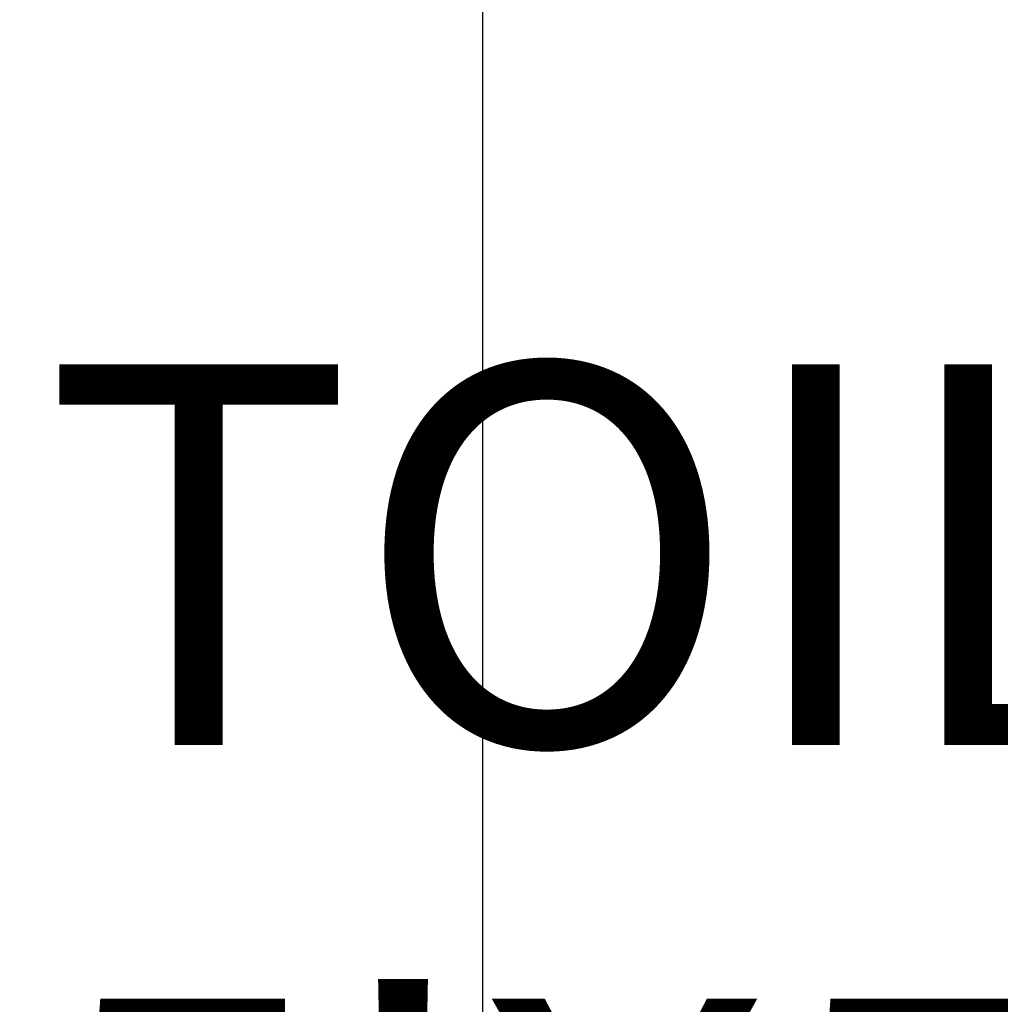
# Model space of a CAD drawing. Units: inches. Extents: x 2696 to 3240, y 1564 to 2310.
# Tile 35 of 76: x 3138 to 3161, y 1722 to 1745. Entities that reach past the tile are written whole.
import ezdxf

# ---------------------------------------------------------------- set-up
doc = ezdxf.new("R2010")
doc.units = ezdxf.units.IN
doc.layers.add('A-ANNO-DIMS', color=3, linetype='Continuous', lineweight=18)
doc.layers.add('A-AREA-IDEN', color=7, linetype='Continuous', lineweight=18)
doc.styles.add('TIMES NEW', font='times.ttf')
doc.styles.add('YQ_DIM', font='SUPEROS.SHX', dxfattribs={"width": 0.8, "bigfont": 'HZDX.SHX'})
doc.dimstyles.new('Siddhuu', dxfattribs={"dimtxt": 6, "dimasz": 2.5, "dimexe": 1.25, "dimexo": 0.625, "dimtad": 1, "dimdec": 1, "dimlunit": 4, "dimtxsty": 'TIMES NEW', "dimcen": 2.5, "dimclrd": 256, "dimclre": 1, "dimclrt": 7, "dimadec": 0, "dimazin": 0, "dimtfac": 1, "dimtdec": 1, "dimtmove": 0, "dimatfit": 3, "dimfxl": 1, "dimtolj": 1, "dimlwd": -1, "dimarcsym": 0})

# ---------------------------------------------------------------- blocks, each defined once
blk = doc.blocks.new('*D51')
at = {"layer": 'A-ANNO-DIMS', "color": 1, "lineweight": -2, "transparency": 16777216}
for p, q in [((3016.611, 1979.576), (3016.611, 1568.951)), ((3148.611, 1979.576), (3148.611, 1568.951))]:
    blk.add_line(p, q, dxfattribs=at)
at = {"layer": 'A-ANNO-DIMS', "transparency": 16777216}
blk.add_line((3019.111, 1570.201), (3146.111, 1570.201), dxfattribs=at)
for points in [[(3019.111, 1570.618), (3019.111, 1569.784), (3016.611, 1570.201)], [(3146.111, 1570.618), (3146.111, 1569.784), (3148.611, 1570.201)]]:
    blk.add_solid(points, dxfattribs=at)
at = {"layer": 'Defpoints', "color": 0, "transparency": 16777216}
for p in [(3016.611, 1980.201), (3148.611, 1980.201), (3148.611, 1570.201)]:
    blk.add_point(p, dxfattribs=at)
at = {"layer": 'A-ANNO-DIMS', "color": 7, "transparency": 16777216, "insert": (3082.611, 1573.878), "char_height": 6, "attachment_point": 5, "style": 'TIMES NEW'}
blk.add_mtext('\\A1;11\'-0"', dxfattribs=at)
blk = doc.blocks.new('*D52')
at = {"layer": 'A-ANNO-DIMS', "color": 1, "lineweight": -2, "transparency": 16777216}
for p, q in [((3148.611, 1979.576), (3148.611, 1568.951)), ((3190.611, 1979.576), (3190.611, 1568.951))]:
    blk.add_line(p, q, dxfattribs=at)
at = {"layer": 'A-ANNO-DIMS', "transparency": 16777216}
blk.add_line((3151.111, 1570.201), (3188.111, 1570.201), dxfattribs=at)
for points in [[(3151.111, 1570.618), (3151.111, 1569.784), (3148.611, 1570.201)], [(3188.111, 1570.618), (3188.111, 1569.784), (3190.611, 1570.201)]]:
    blk.add_solid(points, dxfattribs=at)
at = {"layer": 'Defpoints', "color": 0, "transparency": 16777216}
for p in [(3148.611, 1980.201), (3190.611, 1980.201), (3190.611, 1570.201)]:
    blk.add_point(p, dxfattribs=at)
at = {"layer": 'A-ANNO-DIMS', "color": 7, "transparency": 16777216, "insert": (3169.611, 1573.878), "char_height": 6, "attachment_point": 5, "style": 'TIMES NEW'}
blk.add_mtext('\\A1;3\'-6"', dxfattribs=at)
blk = doc.blocks.new('*D56')
at = {"layer": 'A-ANNO-DIMS', "color": 1, "lineweight": -2, "transparency": 16777216}
for p, q in [((2966.334, 1884.201), (3235.861, 1884.201)), ((2966.334, 1665.201), (3235.861, 1665.201))]:
    blk.add_line(p, q, dxfattribs=at)
at = {"layer": 'A-ANNO-DIMS', "transparency": 16777216}
blk.add_line((3234.611, 1667.701), (3234.611, 1881.701), dxfattribs=at)
for points in [[(3234.195, 1881.701), (3235.028, 1881.701), (3234.611, 1884.201)], [(3234.195, 1667.701), (3235.028, 1667.701), (3234.611, 1665.201)]]:
    blk.add_solid(points, dxfattribs=at)
at = {"layer": 'Defpoints', "color": 0, "transparency": 16777216}
for p in [(2965.709, 1884.201), (3234.611, 1884.201), (2965.709, 1665.201)]:
    blk.add_point(p, dxfattribs=at)
at = {"layer": 'A-ANNO-DIMS', "color": 7, "transparency": 16777216, "insert": (3230.934, 1774.701), "char_height": 6, "attachment_point": 5, "rotation": 90, "style": 'TIMES NEW'}
blk.add_mtext('\\A1;18\'-3"', dxfattribs=at)

msp = doc.modelspace()

# ---------------------------------------------------------------- texts
at = {"layer": 'A-AREA-IDEN', "insert": (3138.221, 1737.206), "char_height": 9, "attachment_point": 1, "style": 'YQ_DIM'}
msp.add_mtext_dynamic_manual_height_columns('TOILET\\P5\'X5\'4.5"', width=48.00324, gutter_width=12.5, heights=[0], dxfattribs=at)

# ---------------------------------------------------------------- dimensions: what is measured, and where the dimension line sits
at = {"layer": 'A-ANNO-DIMS'}
for base, p1, p2, picture, middle in [((3148.611, 1570.201), (3016.611, 1980.201), (3148.611, 1980.201), '*D51', (3082.611, 1573.878)), ((3190.611, 1570.201), (3148.611, 1980.201), (3190.611, 1980.201), '*D52', (3169.611, 1573.878))]:
    dim = msp.add_linear_dim(base=base, p1=p1, p2=p2, dimstyle='Siddhuu', override={"dimdec": 1, "dimlfac": 1, "dimrnd": 0, "dimzin": 1, "dimdsep": 46, "dimlunit": 4, "dimfrac": 2}, dxfattribs=at)
    dim.commit()
    dim.dimension.update_dxf_attribs({"geometry": picture, "text_midpoint": middle})
dim = msp.add_linear_dim(base=(3234.611, 1884.201), p1=(2965.709, 1665.201), p2=(2965.709, 1884.201), angle=90, dimstyle='Siddhuu', override={"dimdec": 1, "dimlfac": 1, "dimrnd": 0, "dimzin": 1, "dimdsep": 46, "dimlunit": 4, "dimfrac": 2}, dxfattribs=at)
dim.commit()
dim.dimension.update_dxf_attribs({"geometry": '*D56', "text_midpoint": (3230.934, 1774.701)})

doc.saveas('drawing.dxf')
